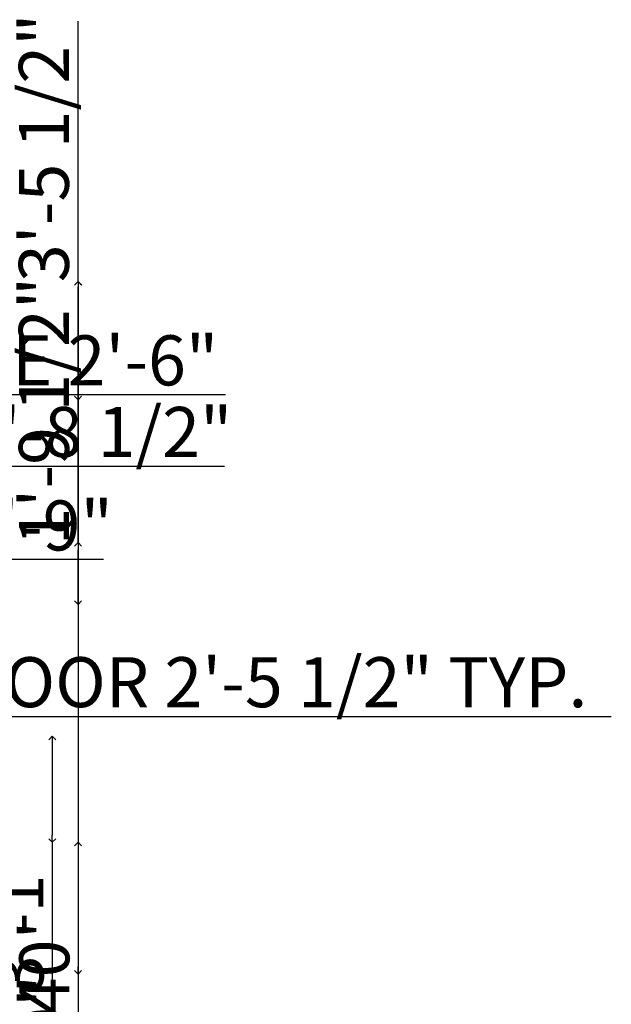
# Model space of a CAD drawing. Units: inches. Extents: x 597 to 1323, y 1833 to 2686.
# Tile 10 of 10: x 1116 to 1323, y 2171 to 2515. Entities that reach past the tile are written whole.
import ezdxf

# ---------------------------------------------------------------- set-up
doc = ezdxf.new("R2010")
doc.units = ezdxf.units.IN
doc.layers.add('A-ANNO-DIMS', color=2, linetype='Continuous', lineweight=18)
doc.styles.get("Standard").update_dxf_attribs({"font": 'arial.ttf'})
doc.dimstyles.new('ISO-25', dxfattribs={"dimtxt": 17.5, "dimasz": 2.5, "dimexe": 0, "dimexo": 0, "dimtad": 1, "dimdec": 1, "dimlunit": 3, "dimtxsty": 'Standard', "dimblk": 'OPEN90', "dimcen": 2.5, "dimadec": 0, "dimazin": 0, "dimtfac": 1, "dimtdec": 1, "dimtmove": 0, "dimatfit": 3, "dimfxl": 0, "dimfxlon": 1, "dimarcsym": 0})

# ---------------------------------------------------------------- blocks, each defined once
blk = doc.blocks.new('_Open90')
at = {"color": 0, "linetype": 'ByBlock', "lineweight": -2}
for p, q in [((0, 0), (-1, 0)), ((-0.5, 0.5), (0, 0)), ((0, 0), (-0.5, -0.5))]:
    blk.add_line(p, q, dxfattribs=at)
blk = doc.blocks.new('*D22')
at = {"layer": 'A-ANNO-DIMS', "color": 0, "lineweight": -2, "transparency": 16777216}
blk.add_line((1136.67, 2421.11), (1136.67, 1946.11), dxfattribs=at)
at = {"layer": 'Defpoints', "color": 0, "transparency": 16777216}
for p in [(1107.89, 2423.61), (1107.89, 1943.61), (1136.67, 1943.61)]:
    blk.add_point(p, dxfattribs=at)
at = {"layer": 'A-ANNO-DIMS', "color": 0, "lineweight": -2, "transparency": 16777216, "xscale": 2.5, "yscale": 2.5, "zscale": 2.5}
for p, rotation in [((1136.67, 2423.61), 90), ((1136.67, 1943.61), 270)]:
    blk.add_blockref('_Open90', p, dxfattribs=dict(at, rotation=rotation))
at = {"layer": 'A-ANNO-DIMS', "color": 0, "transparency": 16777216, "insert": (1127.11, 2183.61), "char_height": 17.5, "attachment_point": 5, "rotation": 90}
blk.add_mtext("40'", dxfattribs=at)
blk = doc.blocks.new('*D37')
at = {"layer": 'A-ANNO-DIMS', "color": 0, "lineweight": -2, "transparency": 16777216}
for p, q in [((975.39, 2271.58), (999.89, 2271.58)), ((1002.39, 2271.58), (1323.28, 2271.58))]:
    blk.add_line(p, q, dxfattribs=at)
at = {"layer": 'Defpoints', "color": 0, "transparency": 16777216}
for p in [(972.89, 2276), (1002.39, 2276), (1002.39, 2271.58)]:
    blk.add_point(p, dxfattribs=at)
at = {"layer": 'A-ANNO-DIMS', "color": 0, "lineweight": -2, "transparency": 16777216, "xscale": 2.5, "yscale": 2.5, "zscale": 2.5, "rotation": 180}
blk.add_blockref('_Open90', (972.89, 2271.58), dxfattribs=at)
at = {"layer": 'A-ANNO-DIMS', "color": 0, "lineweight": -2, "transparency": 16777216, "xscale": 2.5, "yscale": 2.5, "zscale": 2.5}
blk.add_blockref('_Open90', (1002.39, 2271.58), dxfattribs=at)
at = {"layer": 'A-ANNO-DIMS', "color": 0, "transparency": 16777216, "insert": (1164.08, 2281.25), "char_height": 17.5, "attachment_point": 5}
blk.add_mtext('SWING DOOR 2\'-5 1/2" TYP.', dxfattribs=at)
blk = doc.blocks.new('*D48')
at = {"layer": 'A-ANNO-DIMS', "color": 0, "lineweight": -2, "transparency": 16777216}
for p, q in [((1078.41, 2326.5), (1094.41, 2326.5)), ((1096.91, 2326.5), (1145.53, 2326.5))]:
    blk.add_line(p, q, dxfattribs=at)
at = {"layer": 'Defpoints', "color": 0, "transparency": 16777216}
for p in [(1075.91, 2331.9), (1096.91, 2331.9), (1096.91, 2326.5)]:
    blk.add_point(p, dxfattribs=at)
at = {"layer": 'A-ANNO-DIMS', "color": 0, "lineweight": -2, "transparency": 16777216, "xscale": 2.5, "yscale": 2.5, "zscale": 2.5, "rotation": 180}
blk.add_blockref('_Open90', (1075.91, 2326.5), dxfattribs=at)
at = {"layer": 'A-ANNO-DIMS', "color": 0, "lineweight": -2, "transparency": 16777216, "xscale": 2.5, "yscale": 2.5, "zscale": 2.5}
blk.add_blockref('_Open90', (1096.91, 2326.5), dxfattribs=at)
at = {"layer": 'A-ANNO-DIMS', "color": 0, "transparency": 16777216, "insert": (1122.47, 2336.06), "char_height": 17.5, "attachment_point": 5}
blk.add_mtext('1\'-9"', dxfattribs=at)
blk = doc.blocks.new('*D50')
at = {"layer": 'A-ANNO-DIMS', "color": 0, "lineweight": -2, "transparency": 16777216}
for p, q in [((1090.91, 2359.08), (1094.41, 2359.08)), ((1096.91, 2359.08), (1187.96, 2359.08))]:
    blk.add_line(p, q, dxfattribs=at)
at = {"layer": 'Defpoints', "color": 0, "transparency": 16777216}
for p in [(1096.91, 2359.08), (1088.41, 2357.28), (1096.91, 2357.28)]:
    blk.add_point(p, dxfattribs=at)
at = {"layer": 'A-ANNO-DIMS', "color": 0, "lineweight": -2, "transparency": 16777216, "xscale": 2.5, "yscale": 2.5, "zscale": 2.5, "rotation": 180}
blk.add_blockref('_Open90', (1088.41, 2359.08), dxfattribs=at)
at = {"layer": 'A-ANNO-DIMS', "color": 0, "lineweight": -2, "transparency": 16777216, "xscale": 2.5, "yscale": 2.5, "zscale": 2.5}
blk.add_blockref('_Open90', (1096.91, 2359.08), dxfattribs=at)
at = {"layer": 'A-ANNO-DIMS', "color": 0, "transparency": 16777216, "insert": (1143.68, 2368.75), "char_height": 17.5, "attachment_point": 5}
blk.add_mtext('0\'-8 1/2"', dxfattribs=at)
blk = doc.blocks.new('*D53')
at = {"layer": 'A-ANNO-DIMS', "color": 0, "lineweight": -2, "transparency": 16777216}
for p, q in [((1017.66, 2384.11), (1042.66, 2384.11)), ((1045.16, 2384.11), (1188.25, 2384.11))]:
    blk.add_line(p, q, dxfattribs=at)
at = {"layer": 'Defpoints', "color": 0, "transparency": 16777216}
for p in [(1015.16, 2388.61), (1045.16, 2388.61), (1045.16, 2384.11)]:
    blk.add_point(p, dxfattribs=at)
at = {"layer": 'A-ANNO-DIMS', "color": 0, "lineweight": -2, "transparency": 16777216, "xscale": 2.5, "yscale": 2.5, "zscale": 2.5, "rotation": 180}
blk.add_blockref('_Open90', (1015.16, 2384.11), dxfattribs=at)
at = {"layer": 'A-ANNO-DIMS', "color": 0, "lineweight": -2, "transparency": 16777216, "xscale": 2.5, "yscale": 2.5, "zscale": 2.5}
blk.add_blockref('_Open90', (1045.16, 2384.11), dxfattribs=at)
at = {"layer": 'A-ANNO-DIMS', "color": 0, "transparency": 16777216, "insert": (1117.95, 2393.78), "char_height": 17.5, "attachment_point": 5}
blk.add_mtext('RANGE 2\'-6"', dxfattribs=at)
blk = doc.blocks.new('*D64')
at = {"layer": 'A-ANNO-DIMS', "color": 0, "lineweight": -2, "transparency": 16777216}
for p, q in [((1136.64, 2423.61), (1136.64, 2514.65)), ((1136.64, 2384.76), (1136.64, 2421.11))]:
    blk.add_line(p, q, dxfattribs=at)
at = {"layer": 'Defpoints', "color": 0, "transparency": 16777216}
for p in [(1107.89, 2423.61), (1136.64, 2423.61), (1107.89, 2382.26)]:
    blk.add_point(p, dxfattribs=at)
at = {"layer": 'A-ANNO-DIMS', "color": 0, "lineweight": -2, "transparency": 16777216, "xscale": 2.5, "yscale": 2.5, "zscale": 2.5}
for p, rotation in [((1136.64, 2423.61), 90), ((1136.64, 2382.26), 270)]:
    blk.add_blockref('_Open90', p, dxfattribs=dict(at, rotation=rotation))
at = {"layer": 'A-ANNO-DIMS', "color": 0, "transparency": 16777216, "insert": (1126.96, 2470.38), "char_height": 17.5, "attachment_point": 5, "rotation": 90}
blk.add_mtext('3\'-5 1/2"', dxfattribs=at)
blk = doc.blocks.new('*D65')
at = {"layer": 'A-ANNO-DIMS', "color": 0, "lineweight": -2, "transparency": 16777216}
for p, q in [((1136.64, 2225.03), (1136.64, 2183.94)), ((1136.64, 2181.44), (1136.64, 2117.59))]:
    blk.add_line(p, q, dxfattribs=at)
at = {"layer": 'Defpoints', "color": 0, "transparency": 16777216}
for p in [(1107.89, 2227.53), (1107.89, 2181.44), (1136.64, 2181.44)]:
    blk.add_point(p, dxfattribs=at)
at = {"layer": 'A-ANNO-DIMS', "color": 0, "lineweight": -2, "transparency": 16777216, "xscale": 2.5, "yscale": 2.5, "zscale": 2.5}
for p, rotation in [((1136.64, 2227.53), 90), ((1136.64, 2181.44), 270)]:
    blk.add_blockref('_Open90', p, dxfattribs=dict(at, rotation=rotation))
at = {"layer": 'A-ANNO-DIMS', "color": 0, "transparency": 16777216, "insert": (1127.07, 2148.27), "char_height": 17.5, "attachment_point": 5, "rotation": 90}
blk.add_mtext('3\'-10"', dxfattribs=at)
blk = doc.blocks.new('*D73')
at = {"layer": 'A-ANNO-DIMS', "color": 0, "lineweight": -2, "transparency": 16777216}
for p, q in [((1136.64, 2332.34), (1136.64, 2421.74)), ((1136.64, 2313.23), (1136.64, 2329.84))]:
    blk.add_line(p, q, dxfattribs=at)
at = {"layer": 'Defpoints', "color": 0, "transparency": 16777216}
for p in [(1096.47, 2332.34), (1136.64, 2332.34), (1098.89, 2310.73)]:
    blk.add_point(p, dxfattribs=at)
at = {"layer": 'A-ANNO-DIMS', "color": 0, "lineweight": -2, "transparency": 16777216, "xscale": 2.5, "yscale": 2.5, "zscale": 2.5}
for p, rotation in [((1136.64, 2332.34), 90), ((1136.64, 2310.73), 270)]:
    blk.add_blockref('_Open90', p, dxfattribs=dict(at, rotation=rotation))
at = {"layer": 'A-ANNO-DIMS', "color": 0, "transparency": 16777216, "insert": (1126.96, 2378.29), "char_height": 17.5, "attachment_point": 5, "rotation": 90}
blk.add_mtext('1\'-9 1/2"', dxfattribs=at)
blk = doc.blocks.new('*D74')
at = {"layer": 'A-ANNO-DIMS', "color": 0, "lineweight": -2, "transparency": 16777216}
for p, q in [((1127.64, 2262.11), (1127.64, 2230.03)), ((1127.64, 2227.53), (1127.64, 2177.27))]:
    blk.add_line(p, q, dxfattribs=at)
at = {"layer": 'Defpoints', "color": 0, "transparency": 16777216}
for p in [(1098.89, 2264.61), (1098.89, 2227.53), (1127.64, 2227.53)]:
    blk.add_point(p, dxfattribs=at)
at = {"layer": 'A-ANNO-DIMS', "color": 0, "lineweight": -2, "transparency": 16777216, "xscale": 2.5, "yscale": 2.5, "zscale": 2.5}
for p, rotation in [((1127.64, 2264.61), 90), ((1127.64, 2227.53), 270)]:
    blk.add_blockref('_Open90', p, dxfattribs=dict(at, rotation=rotation))
at = {"layer": 'A-ANNO-DIMS', "color": 0, "transparency": 16777216, "insert": (1118.07, 2201.15), "char_height": 17.5, "attachment_point": 5, "rotation": 90}
blk.add_mtext('3\'-1"', dxfattribs=at)

msp = doc.modelspace()

# ---------------------------------------------------------------- dimensions: what is measured, and where the dimension line sits
at = {"layer": 'A-ANNO-DIMS'}
for base, p1, p2, angle, override, picture, middle in [((1136.6363, 2423.6106), (1107.8863, 2382.26), (1107.8863, 2423.6106), 90, {"dimdec": 1, "dimlfac": 1, "dimrnd": 0, "dimzin": 1, "dimdsep": 46, "dimlunit": 4, "dimfrac": 2}, '*D64', (1126.9569, 2470.3782)), ((1136.64, 2332.34), (1098.89, 2310.73), (1096.47, 2332.34), 90, {"dimdec": 1, "dimlfac": 1, "dimrnd": 0, "dimzin": 1, "dimdsep": 46, "dimlunit": 4, "dimfrac": 2}, '*D73', (1126.96, 2378.29)), ((1136.67, 1943.61), (1107.89, 2423.61), (1107.89, 1943.61), 90, {"dimclrd": 0, "dimclre": 0, "dimclrt": 0}, '*D22', (1127.11, 2183.61)), ((1127.64, 2227.53), (1098.89, 2264.61), (1098.89, 2227.53), 270, {"dimdec": 1, "dimlfac": 1, "dimrnd": 0, "dimzin": 1, "dimdsep": 46, "dimlunit": 4, "dimfrac": 2}, '*D74', (1118.07, 2201.15)), ((1136.64, 2181.44), (1107.89, 2227.53), (1107.89, 2181.44), 90, {"dimdec": 1, "dimlfac": 1, "dimrnd": 0, "dimzin": 1, "dimdsep": 46, "dimlunit": 4, "dimfrac": 2}, '*D65', (1127.07, 2148.27))]:
    dim = msp.add_linear_dim(base=base, p1=p1, p2=p2, angle=angle, dimstyle='ISO-25', override=override, dxfattribs=at)
    dim.commit()
    dim.dimension.update_dxf_attribs({"geometry": picture, "text_midpoint": middle})
for base, p1, p2, text, picture, middle in [((1045.16, 2384.11), (1015.16, 2388.61), (1045.16, 2388.61), 'RANGE <>', '*D53', (1117.95, 2393.78)), ((1002.39, 2271.58), (972.89, 2276), (1002.39, 2276), 'SWING DOOR <> TYP.', '*D37', (1164.08, 2281.25))]:
    dim = msp.add_linear_dim(base=base, p1=p1, p2=p2, text=text, dimstyle='ISO-25', override={"dimdec": 1, "dimlfac": 1, "dimrnd": 0, "dimzin": 1, "dimdsep": 46, "dimlunit": 4, "dimfrac": 2}, dxfattribs=at)
    dim.commit()
    dim.dimension.update_dxf_attribs({"geometry": picture, "text_midpoint": middle})
for base, p1, p2, picture, middle in [((1096.91, 2359.08), (1088.41, 2357.28), (1096.91, 2357.28), '*D50', (1143.68, 2368.75)), ((1096.91, 2326.5), (1075.91, 2331.9), (1096.91, 2331.9), '*D48', (1122.47, 2336.06))]:
    dim = msp.add_linear_dim(base=base, p1=p1, p2=p2, dimstyle='ISO-25', override={"dimdec": 1, "dimlfac": 1, "dimrnd": 0, "dimzin": 1, "dimdsep": 46, "dimlunit": 4, "dimfrac": 2}, dxfattribs=at)
    dim.commit()
    dim.dimension.update_dxf_attribs({"geometry": picture, "text_midpoint": middle})

doc.saveas('drawing.dxf')
